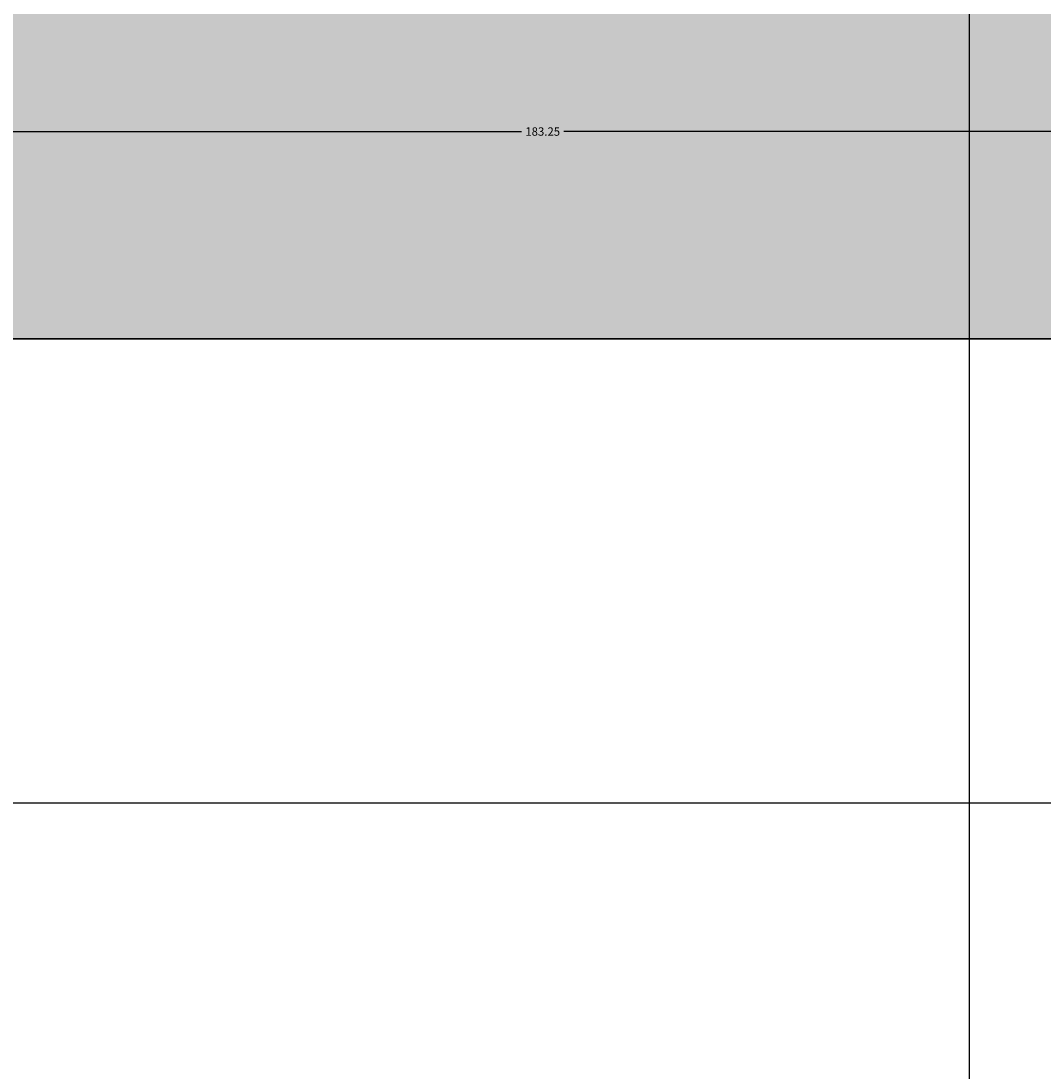
# Model space of a CAD drawing. Units: inches. Extents: x -1 to 292, y -3 to 199.
# Tile 16 of 52: x 102 to 124, y 20 to 42. Entities that reach past the tile are written whole.
import ezdxf

# ---------------------------------------------------------------- set-up
doc = ezdxf.new("R2010")
doc.units = ezdxf.units.IN
doc.header["$MEASUREMENT"] = 0
for name, color, linetype, lineweight in [('M-DIMS', 2, 'Continuous', 18), ('M-EQPM', 7, 'Continuous', 35), ('M-PATT', 8, 'Continuous', 13)]:
    doc.layers.add(name, color=color, linetype=linetype, lineweight=lineweight)
doc.styles.get("Standard").update_dxf_attribs({"font": 'arial.ttf'})
doc.dimstyles.get("Standard").update_dxf_attribs({"dimtxt": 0.18, "dimasz": 0.18, "dimexe": 0.18, "dimexo": 0.0625, "dimgap": 0.09, "dimtad": 0, "dimtih": 1, "dimtoh": 1, "dimdec": 4, "dimzin": 0, "dimdsep": 46, "dimtxsty": 'Standard', "dimcen": 0.09, "dimadec": 0, "dimazin": 0, "dimtfac": 1, "dimtdec": 4, "dimtofl": 0, "dimtmove": 0, "dimatfit": 3, "dimfxl": 1, "dimtolj": 1, "dimtzin": 0, "dimarcsym": 0})

# ---------------------------------------------------------------- blocks, each defined once
blk = doc.blocks.new('*D7')
at = {"layer": 'Defpoints', "color": 0, "transparency": 16777216}
for p in [(21.861, 54.582), (205.115, 54.582), (21.861, 39.982)]:
    blk.add_point(p, dxfattribs=at)
at = {"layer": 'M-DIMS', "color": 0, "lineweight": -2, "transparency": 16777216}
for p, q in [((21.861, 54.52), (21.861, 39.802)), ((205.115, 54.52), (205.115, 39.802)), ((22.041, 39.982), (113.033, 39.982)), ((204.935, 39.982), (113.944, 39.982))]:
    blk.add_line(p, q, dxfattribs=at)
at = {"layer": 'M-DIMS', "color": 0, "transparency": 16777216}
for points in [[(22.041, 40.012), (22.041, 39.952), (21.861, 39.982)], [(204.935, 40.012), (204.935, 39.952), (205.115, 39.982)]]:
    blk.add_solid(points, dxfattribs=at)
at = {"layer": 'M-DIMS', "color": 0, "transparency": 16777216, "insert": (113.488, 39.982), "char_height": 0.18, "attachment_point": 5}
blk.add_mtext('\\A1;183.25', dxfattribs=at)
blk = doc.blocks.new('*D8')
at = {"layer": 'Defpoints', "color": 0, "transparency": 16777216}
for p in [(-0.662, 126.765), (111.488, 126.765), (69.013, 25.514)]:
    blk.add_point(p, dxfattribs=at)
at = {"layer": 'M-DIMS', "color": 0, "lineweight": -2, "transparency": 16777216}
for p, q in [((111.426, 126.765), (-0.842, 126.765)), ((-0.662, 126.585), (-0.662, 76.321)), ((-0.662, 25.694), (-0.662, 75.958)), ((68.951, 25.514), (-0.842, 25.514))]:
    blk.add_line(p, q, dxfattribs=at)
at = {"layer": 'M-DIMS', "color": 0, "transparency": 16777216}
for points in [[(-0.692, 126.585), (-0.632, 126.585), (-0.662, 126.765)], [(-0.692, 25.694), (-0.632, 25.694), (-0.662, 25.514)]]:
    blk.add_solid(points, dxfattribs=at)
at = {"layer": 'M-DIMS', "color": 0, "transparency": 16777216, "insert": (-0.662, 76.14), "char_height": 0.18, "attachment_point": 5}
blk.add_mtext('\\A1;101.25', dxfattribs=at)
blk = doc.blocks.new('*D11')
at = {"layer": 'Defpoints', "color": 0, "transparency": 16777216}
for p in [(79.013, 35.514), (292.04, 35.514), (79.013, 25.514)]:
    blk.add_point(p, dxfattribs=at)
at = {"layer": 'M-DIMS', "color": 0, "lineweight": -2, "transparency": 16777216}
for p, q in [((79.076, 35.514), (292.22, 35.514)), ((292.04, 35.334), (292.04, 30.696)), ((292.04, 25.694), (292.04, 30.332)), ((79.076, 25.514), (292.22, 25.514))]:
    blk.add_line(p, q, dxfattribs=at)
at = {"layer": 'M-DIMS', "color": 0, "transparency": 16777216}
for points in [[(292.01, 35.334), (292.07, 35.334), (292.04, 35.514)], [(292.01, 25.694), (292.07, 25.694), (292.04, 25.514)]]:
    blk.add_solid(points, dxfattribs=at)
at = {"layer": 'M-DIMS', "color": 0, "transparency": 16777216, "insert": (292.04, 30.514), "char_height": 0.18, "attachment_point": 5}
blk.add_mtext('\\A1;10', dxfattribs=at)
blk = doc.blocks.new('*D13')
at = {"layer": 'Defpoints', "color": 0, "transparency": 16777216}
for p in [(79.013, 25.514), (148.429, 25.514), (79.013, 10.914)]:
    blk.add_point(p, dxfattribs=at)
at = {"layer": 'M-DIMS', "color": 0, "lineweight": -2, "transparency": 16777216}
for p, q in [((79.013, 25.452), (79.013, 10.734)), ((148.429, 25.452), (148.429, 10.734)), ((79.193, 10.914), (113.328, 10.914)), ((148.249, 10.914), (114.115, 10.914))]:
    blk.add_line(p, q, dxfattribs=at)
at = {"layer": 'M-DIMS', "color": 0, "transparency": 16777216}
for points in [[(79.193, 10.944), (79.193, 10.884), (79.013, 10.914)], [(148.249, 10.944), (148.249, 10.884), (148.429, 10.914)]]:
    blk.add_solid(points, dxfattribs=at)
at = {"layer": 'M-DIMS', "color": 0, "transparency": 16777216, "insert": (113.721, 10.914), "char_height": 0.18, "attachment_point": 5}
blk.add_mtext('\\A1;69.42', dxfattribs=at)
blk = doc.blocks.new('*D22')
at = {"layer": 'Defpoints', "color": 0, "transparency": 16777216}
for p in [(82.679, 51.267), (122.679, 51.267), (122.679, -2.71)]:
    blk.add_point(p, dxfattribs=at)
at = {"layer": 'M-DIMS', "color": 0, "lineweight": -2, "transparency": 16777216}
for p, q in [((82.679, 51.205), (82.679, -2.89)), ((122.679, 51.205), (122.679, -2.89)), ((82.859, -2.71), (102.457, -2.71)), ((122.499, -2.71), (102.901, -2.71))]:
    blk.add_line(p, q, dxfattribs=at)
at = {"layer": 'M-DIMS', "color": 0, "transparency": 16777216}
for points in [[(82.859, -2.68), (82.859, -2.74), (82.679, -2.71)], [(122.499, -2.68), (122.499, -2.74), (122.679, -2.71)]]:
    blk.add_solid(points, dxfattribs=at)
at = {"layer": 'M-DIMS', "color": 0, "transparency": 16777216, "insert": (102.679, -2.71), "char_height": 0.18, "attachment_point": 5}
blk.add_mtext('\\A1;40', dxfattribs=at)

msp = doc.modelspace()

# ---------------------------------------------------------------- hatches: boundary and pattern name
at = {"layer": 'M-PATT'}
h = msp.add_hatch(color=256, dxfattribs=at)
h.set_gradient(color1=(0, 255, 255), color2=(0, 255, 255), tint=1)
h.paths.add_polyline_path([(75.3521, 99.7735), (72.66, 101.3278), (70.2665, 99.7735), (67.5744, 101.3278), (65.1809, 99.7735), (62.4888, 101.3278), (60.0953, 99.7735), (57.4032, 101.3278), (55.0097, 99.7735), (52.3176, 101.3278), (49.9241, 99.7735, 0.4142136), (57.8007, 91.897), (61.6788, 91.897), (61.6788, 51.2672), (57.8007, 51.2672, 0.8088808), (54.5813, 36.2021), (65.0947, 51.2672), (64.6788, 51.2672), (64.6788, 91.897), (67.6788, 91.897), (67.6788, 51.2672), (65.0947, 51.2672), (54.5813, 36.2021, 0.1056561), (57.8007, 35.5141), (169.176, 35.5141, 1), (169.176, 51.2672), (162.6788, 51.2672), (162.6788, 91.897), (169.176, 91.897, 0.4144629), (177.0526, 99.7802), (174.372, 101.3278), (171.9786, 99.7735), (169.2864, 101.3278), (166.893, 99.7735), (164.2008, 101.3278), (162.1623, 100.004), (162.1623, 96.1027), (160.6222, 96.1027), (160.6222, 100.4578), (159.1152, 101.3278), (156.7218, 99.7735), (154.0296, 101.3278), (151.6362, 99.7735), (148.944, 101.3278), (146.5506, 99.7735), (143.8584, 101.3278), (141.465, 99.7735), (138.7728, 101.3278), (136.3794, 99.7735), (133.6872, 101.3278), (131.2938, 99.7735), (128.6016, 101.3278), (126.2082, 99.7735), (123.516, 101.3278), (121.1225, 99.7735), (118.4304, 101.3278), (116.0369, 99.7735), (113.3448, 101.3278), (110.9513, 99.7735), (108.2592, 101.3278), (105.8657, 99.7735), (103.1736, 101.3278), (100.7801, 99.7735), (98.088, 101.3278), (95.6945, 99.7735), (93.0024, 101.3278), (90.6089, 99.7735), (87.9168, 101.3278), (85.5233, 99.7735), (82.8312, 101.3278), (80.4377, 99.7735), (77.7456, 101.3278)])
h.paths.add_polyline_path([(79.6788, 91.897), (79.6788, 51.2672), (76.6788, 51.2672), (76.6788, 91.897)], flags=16)
h.paths.add_polyline_path([(73.6788, 91.897), (73.6788, 51.2672), (70.6788, 51.2672), (70.6788, 91.897)], flags=16)
h.paths.add_polyline_path([(82.6788, 91.897), (101.6788, 91.897), (101.6788, 51.2672), (82.6788, 51.2672)], flags=16)
h.paths.add_polyline_path([(104.6788, 91.897), (107.6788, 91.897), (107.6788, 51.2672), (104.6788, 51.2672)], flags=16)
h.paths.add_polyline_path([(110.6788, 91.897), (113.6788, 91.897), (113.6788, 51.2672), (110.6788, 51.2672)], flags=16)
h.paths.add_polyline_path([(116.6788, 91.897), (119.6788, 91.897), (119.6788, 51.2672), (116.6788, 51.2672)], flags=16)
h.paths.add_polyline_path([(122.6788, 91.897), (141.6788, 91.897), (141.6788, 51.2672), (144.6788, 51.2672), (144.6788, 91.897), (147.6788, 91.897), (147.6788, 51.2672), (122.6788, 51.2672)], flags=16)
h.paths.add_polyline_path([(150.6788, 91.897), (153.6788, 91.897), (153.6788, 51.2672), (150.6788, 51.2672)], flags=16)
h.paths.add_polyline_path([(156.6788, 91.897), (159.6788, 91.897), (159.6788, 51.2672), (156.6788, 51.2672)], flags=16)

# ---------------------------------------------------------------- linework, layer by layer
at = {"layer": 'M-EQPM'}
msp.add_lwpolyline([(61.6788, 51.2672), (57.8007, 51.2672, 1), (57.8007, 35.5141), (169.176, 35.5141, 1), (169.176, 51.2672), (162.6788, 51.2672)], format="xyb", dxfattribs=at)

# ---------------------------------------------------------------- dimensions: what is measured, and where the dimension line sits
at = {"layer": 'M-DIMS'}
for base, p1, p2, angle, override, picture, middle in [((-0.6625, 126.765), (69.013, 25.5141), (111.4883, 126.765), 90, {"dimdec": 2, "dimlfac": 1, "dimrnd": 0, "dimzin": 0, "dimdsep": 46, "dimlunit": 2}, '*D8', (-0.6625, 76.1396)), ((21.8612, 39.9821), (205.1155, 54.5821), (21.8612, 54.5821), 180, {"dimdec": 2, "dimlfac": 1, "dimrnd": 0, "dimzin": 0, "dimdsep": 46, "dimlunit": 2}, '*D7', (113.4883, 39.9821)), ((292.0399, 35.5141), (79.013, 25.5141), (79.013, 35.5141), 90, {"dimdec": 0, "dimlfac": 1, "dimrnd": 0, "dimzin": 0, "dimdsep": 46, "dimlunit": 2}, '*D11', (292.0399, 30.5141)), ((79.013, 10.9141), (148.4295, 25.5141), (79.013, 25.5141), 180, {"dimdec": 2, "dimlfac": 1, "dimrnd": 0, "dimzin": 0, "dimdsep": 46, "dimlunit": 2}, '*D13', (113.7212, 10.9141))]:
    dim = msp.add_linear_dim(base=base, p1=p1, p2=p2, angle=angle, dimstyle='Standard', override=override, dxfattribs=at)
    dim.commit()
    dim.dimension.update_dxf_attribs({"geometry": picture, "text_midpoint": middle})
dim = msp.add_linear_dim(base=(122.6788, -2.7104), p1=(82.6788, 51.2672), p2=(122.6788, 51.2672), dimstyle='Standard', override={"dimdec": 0, "dimlfac": 1, "dimrnd": 0, "dimzin": 0, "dimdsep": 46, "dimlunit": 2}, dxfattribs=at)
dim.commit()
dim.dimension.update_dxf_attribs({"geometry": '*D22', "text_midpoint": (102.6788, -2.7104)})

doc.saveas('drawing.dxf')
